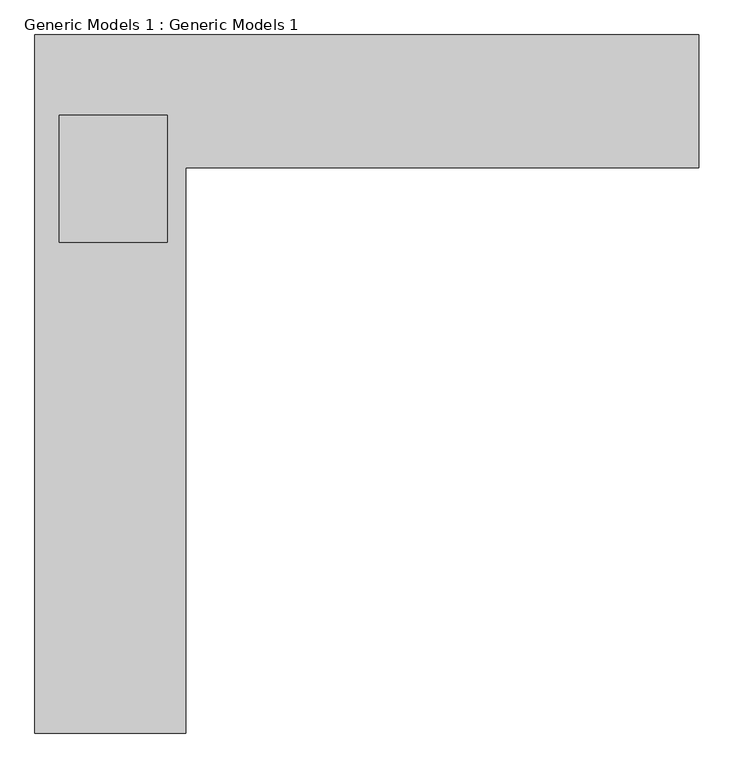
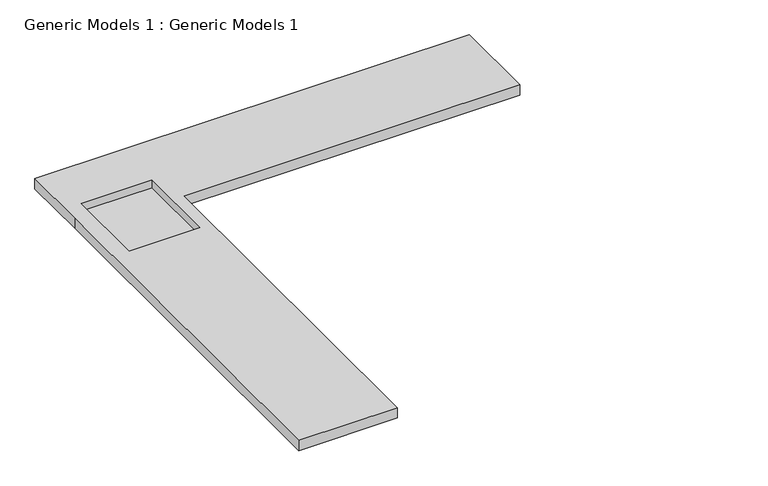
"""IFC4 building model written with IfcOpenShell, lengths in millimetres: proxy geometry, Generic Models 1 : Generic Models 1."""

from ifc_helpers import new_model, si_unit, origin, place, context, project, spatial, faceted_brep, source, transform, mapped, element, save


def generic_models_1_generic_models_1_627619a8(model_context):
    return source(origin(), model_context, "Body", "Brep", [
        faceted_brep([(-10023.2536634, 8025.893892, 1066.8), (-6980.9914732, 8025.893892, 1066.8), (-6980.9914732, 7416.293892, 1066.8), (-9332.7095842, 7416.293892, 1066.8), (-9332.7095842, 4826.0804551, 1066.8), (-10023.2536634, 4826.0804551, 1066.8), (-10023.2536634, 7545.6218675, 1066.8), (-10023.2536634, 8025.893892, 1143.0), (-10023.2536634, 7545.6218675, 1143.0), (-10023.2536634, 4826.0804551, 1143.0), (-9332.7095842, 4826.0804551, 1143.0), (-9332.7095842, 7416.293892, 1143.0), (-6980.9914732, 7416.293892, 1143.0), (-6980.9914732, 8025.893892, 1143.0), (-9912.3896943, 7076.0222021, 1143.0), (-9912.3896943, 7658.0222021, 1143.0), (-9416.3896943, 7658.0222021, 1143.0), (-9416.3896943, 7076.0222021, 1143.0), (-9912.3896943, 7658.0222021, 1085.1684031), (-9912.3896943, 7076.0222021, 1085.1684031), (-9416.3896943, 7076.0222021, 1085.1684031), (-9416.3896943, 7658.0222021, 1085.1684031)], [[[0, 1, 2, 3, 4, 5, 6]], [[7, 8, 9, 10, 11, 12, 13], [14, 15, 16, 17]], [[0, 6, 8, 7]], [[6, 5, 9, 8]], [[5, 4, 10, 9]], [[4, 3, 11, 10]], [[3, 2, 12, 11]], [[2, 1, 13, 12]], [[1, 0, 7, 13]], [[18, 19, 20, 21]], [[19, 18, 15, 14]], [[20, 19, 14, 17]], [[21, 20, 17, 16]], [[18, 21, 16, 15]]]),
    ])


if __name__ == "__main__":
    model = new_model("IFC4")
    model_context = context("Model", 3, world=origin())
    ifc_project = project(units=[si_unit("LENGTHUNIT", "METRE", prefix="MILLI")], contexts=[model_context])
    site = spatial("IfcSite", under=ifc_project)
    building = spatial("IfcBuilding", under=site)
    placement = place(None, origin())
    generic_models_1_generic_models_1_shape = generic_models_1_generic_models_1_627619a8(model_context)
    element("IfcBuildingElementProxy", 1, Name="Generic Models 1 : Generic Models 1", ObjectType="Generic Models 1 : Generic Models 1", at=placement, inside=building, context=model_context, shape_type="MappedRepresentation", body=[
        mapped(generic_models_1_generic_models_1_shape, transform((0.0, 0.0, 0.0), x_axis=(1.0, 0.0, 0.0), y_axis=(0.0, 1.0, 0.0), z_axis=(0.0, 0.0, 1.0))),
    ])
    save(model, "model.ifc")

# Revit data of these elements
# Element 1 (IfcBuildingElementProxy, "Generic Models 1 : Generic Models 1")
#   Materials on its faces: "Concrete, Cast-in-Place, Gray"
# Materials
#   "Concrete, Cast-in-Place, Gray": class "Concrete", colour RGB 192 192 192, transparency 0, Description = "Cast-in-place concrete", Cost = 0
